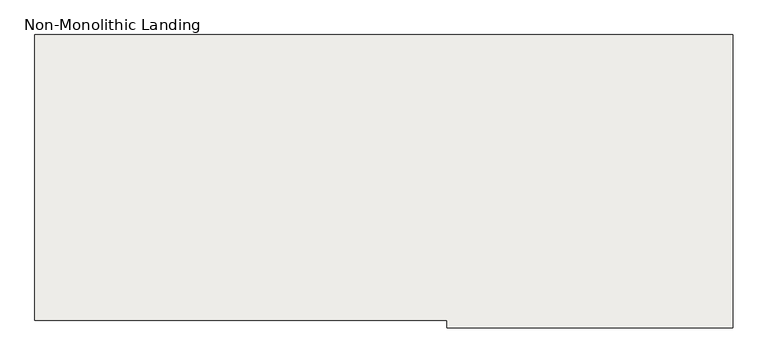
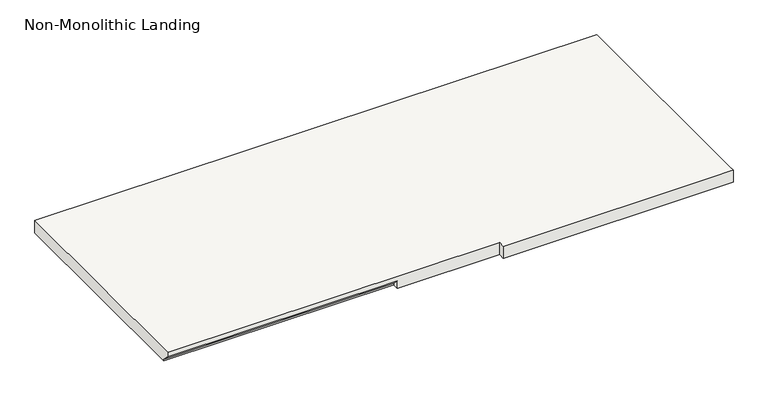
"""IFC4 building model written with IfcOpenShell, lengths in millimetres: slab geometry, Non-Monolithic Landing."""

from ifc_helpers import new_model, si_unit, origin, place, context, project, spatial, faceted_brep, source, transform, mapped, element, save


def non_monolithic_landing_15cb0957(model_context):
    return source(origin(), model_context, "Body", "Brep", [
        faceted_brep([(-3617.4415084, -19522.1851539, 51970.2339133), (-3617.4415084, -19496.7851539, 51944.8339133), (-2703.0415084, -19496.7851539, 51944.8339133), (-2703.0415084, -19522.1851539, 51970.2339133), (-2296.6415084, -19522.1851539, 51989.2839133), (-2296.6415084, -19547.5851539, 51989.2839133), (-1382.2415084, -19547.5851539, 51989.2839133), (-1382.2415084, -19522.1851539, 51989.2839133), (-1382.2415084, -18607.7851539, 51989.2839133), (-3617.4415084, -18607.7851539, 51989.2839133), (-3617.4415084, -19522.1851539, 51989.2839133), (-2703.0415084, -19496.7851539, 51938.4839133), (-3617.4415084, -19496.7851539, 51938.4839133), (-3617.4415084, -18607.7851539, 51938.4839133), (-1382.2415084, -18607.7851539, 51938.4839133), (-1382.2415084, -19522.1851539, 51938.4839133), (-1382.2415084, -19547.5851539, 51938.4839133), (-2296.6415084, -19547.5851539, 51938.4839133), (-2296.6415084, -19522.1851539, 51938.4839133), (-2703.0415084, -19522.1851539, 51938.4839133)], [[[0, 1, 2, 3]], [[4, 5, 6, 7, 8, 9, 10]], [[11, 12, 13, 14, 15, 16, 17, 18, 19]], [[12, 11, 2, 1]], [[11, 19, 3, 2]], [[4, 10, 0, 3, 19, 18]], [[5, 4, 18, 17]], [[6, 5, 17, 16]], [[7, 6, 16, 15]], [[8, 7, 15, 14]], [[9, 8, 14, 13]], [[10, 9, 13, 12, 1, 0]]]),
    ])


if __name__ == "__main__":
    model = new_model("IFC4")
    model_context = context("Model", 3, world=origin())
    ifc_project = project(units=[si_unit("LENGTHUNIT", "METRE", prefix="MILLI")], contexts=[model_context])
    site = spatial("IfcSite", under=ifc_project)
    building = spatial("IfcBuilding", under=site)
    placement = place(None, origin())
    non_monolithic_landing_shape = non_monolithic_landing_15cb0957(model_context)
    element("IfcSlab", 1, ObjectType="Non-Monolithic Landing", at=placement, inside=building, context=model_context, shape_type="MappedRepresentation", body=[
        mapped(non_monolithic_landing_shape, transform((0.0, 0.0, 0.0), x_axis=(1.0, 0.0, 0.0), y_axis=(0.0, 1.0, 0.0), z_axis=(0.0, 0.0, 1.0))),
    ])
    save(model, "model.ifc")
